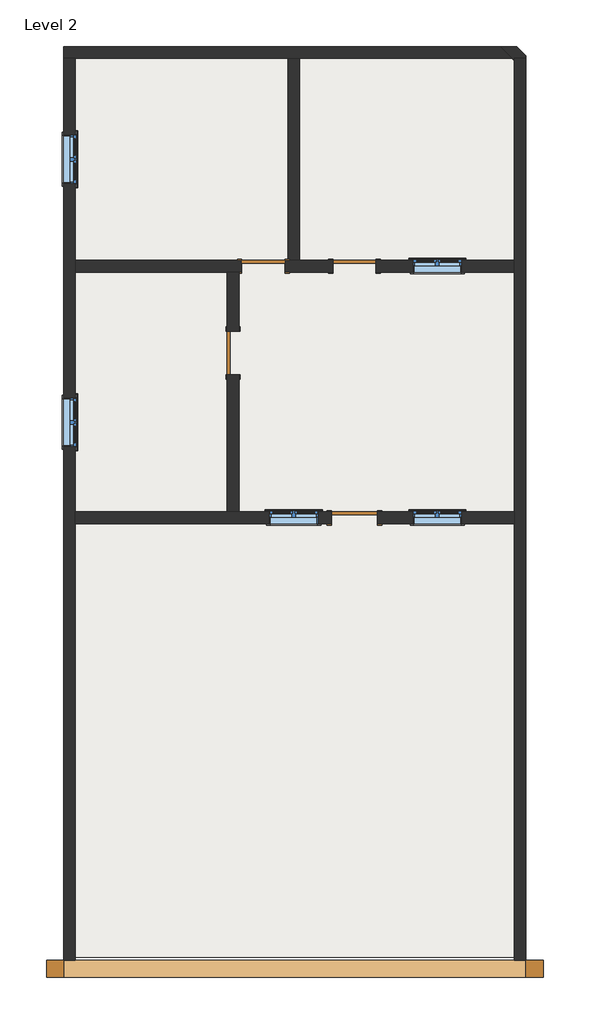
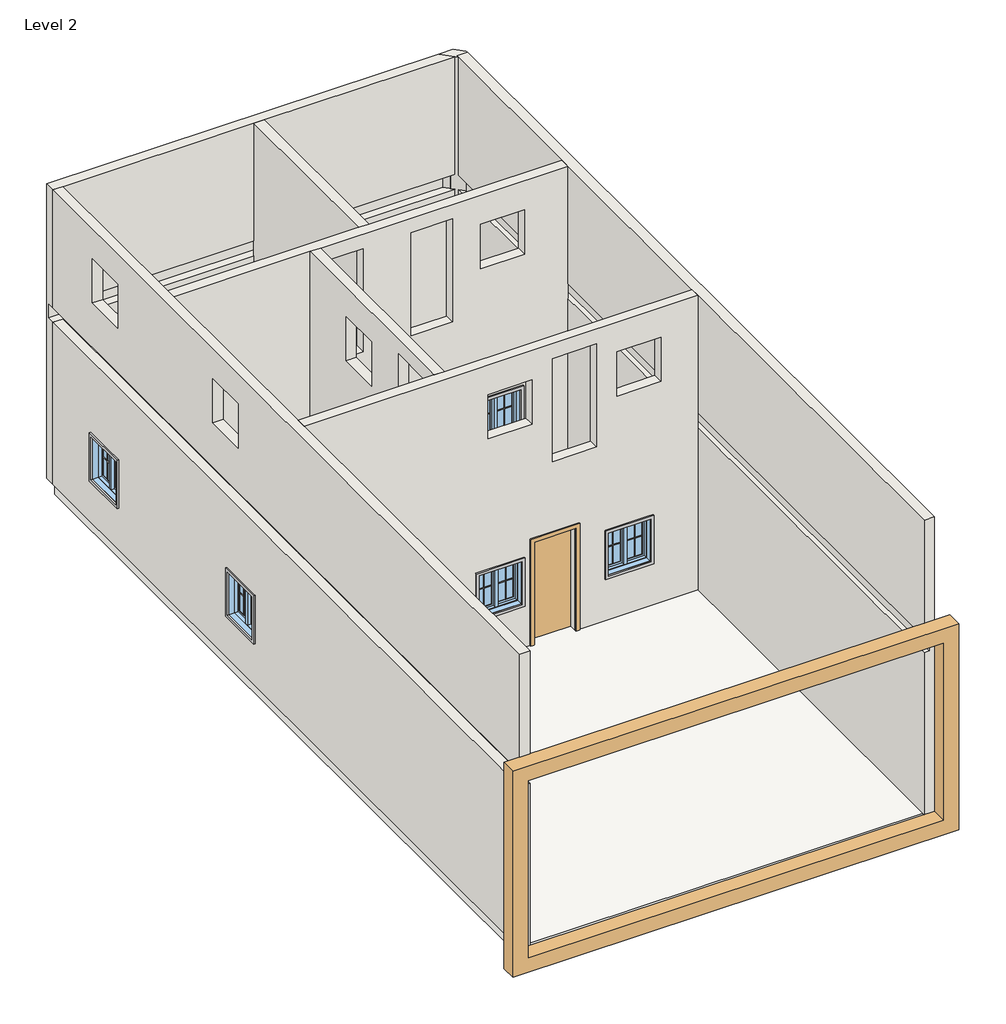
# One storey: 20 proxies, 8 walls, 5 doors, 5 windows, 1 slab.
"""IFC4 building model written with IfcOpenShell, lengths in millimetres."""

from ifc_helpers import new_model, si_unit, frame, origin, place, context, project, spatial, polyline, outline, extrude, faceted_brep, transform, mapped, element, save
from components import muntin_pattern_2x2_muntin_pattern_2x2_b3fe6957, muntin_pattern_2x2_muntin_pattern_2x2_3e0ecaf2, trim_window_exterior_flat_with_sill_41619996, trim_window_interior_flat_picture_frame_51c85655, doors_1_doors_1_af7bef9e, door_fadea3f2, door_64d5ae29, window_c29befe5

model = new_model("IFC4")

# Units and contexts
model_context = context("Model", 3, world=origin())
ifc_project = project(units=[si_unit("LENGTHUNIT", "METRE", prefix="MILLI")], contexts=[model_context])

# Site, building, storey
site = spatial("IfcSite", under=ifc_project)
building = spatial("IfcBuilding", under=site)
storey = spatial("IfcBuildingStorey", under=building, Name="Level 2", Elevation=9144.0)

# Proxies
placement = place(None, origin())
muntin_pattern_2x2_muntin_pattern_2x2_shape = muntin_pattern_2x2_muntin_pattern_2x2_b3fe6957(model_context)
element("IfcBuildingElementProxy", 1, Name="Muntin Pattern_2x2 : Muntin Pattern_2x2", ObjectType="Muntin Pattern_2x2 : Muntin Pattern_2x2", at=placement, inside=storey, context=model_context, shape_type="MappedRepresentation", body=[
    mapped(muntin_pattern_2x2_muntin_pattern_2x2_shape, transform((-9669.8723431, 12327.0201951, 10128.25), x_axis=(1.0, 0.0, 0.0), y_axis=(0.0, 1.0, 0.0), z_axis=(0.0, 0.0, 1.0))),
])
element("IfcBuildingElementProxy", 2, Name="Muntin Pattern_2x2 : Muntin Pattern_2x2", ObjectType="Muntin Pattern_2x2 : Muntin Pattern_2x2", at=placement, inside=storey, context=model_context, shape_type="MappedRepresentation", body=[
    mapped(muntin_pattern_2x2_muntin_pattern_2x2_shape, transform((-15829.9638186, 14328.8576951, 10128.25), x_axis=(0.0, -1.0, 0.0), y_axis=(1.0, 0.0, 0.0), z_axis=(0.0, 0.0, 1.0))),
])
element("IfcBuildingElementProxy", 3, Name="Muntin Pattern_2x2 : Muntin Pattern_2x2", ObjectType="Muntin Pattern_2x2 : Muntin Pattern_2x2", at=placement, inside=storey, context=model_context, shape_type="MappedRepresentation", body=[
    mapped(muntin_pattern_2x2_muntin_pattern_2x2_shape, transform((-15829.9638186, 9706.0576951, 10128.25), x_axis=(0.0, -1.0, 0.0), y_axis=(1.0, 0.0, 0.0), z_axis=(0.0, 0.0, 1.0))),
])
element("IfcBuildingElementProxy", 4, Name="Muntin Pattern_2x2 : Muntin Pattern_2x2", ObjectType="Muntin Pattern_2x2 : Muntin Pattern_2x2", at=placement, inside=storey, context=model_context, shape_type="MappedRepresentation", body=[
    mapped(muntin_pattern_2x2_muntin_pattern_2x2_shape, transform((-12194.9933676, 7907.4201951, 10128.25), x_axis=(1.0, 0.0, 0.0), y_axis=(0.0, 1.0, 0.0), z_axis=(0.0, 0.0, 1.0))),
])
element("IfcBuildingElementProxy", 5, Name="Muntin Pattern_2x2 : Muntin Pattern_2x2", ObjectType="Muntin Pattern_2x2 : Muntin Pattern_2x2", at=placement, inside=storey, context=model_context, shape_type="MappedRepresentation", body=[
    mapped(muntin_pattern_2x2_muntin_pattern_2x2_shape, transform((-9669.8723431, 7907.4201951, 10128.25), x_axis=(1.0, 0.0, 0.0), y_axis=(0.0, 1.0, 0.0), z_axis=(0.0, 0.0, 1.0))),
])
muntin_pattern_2x2_muntin_pattern_2x2_2_shape = muntin_pattern_2x2_muntin_pattern_2x2_3e0ecaf2(model_context)
element("IfcBuildingElementProxy", 6, Name="Muntin Pattern_2x2 : Muntin Pattern_2x2", ObjectType="Muntin Pattern_2x2 : Muntin Pattern_2x2", at=placement, inside=storey, context=model_context, shape_type="MappedRepresentation", body=[
    mapped(muntin_pattern_2x2_muntin_pattern_2x2_2_shape, transform((-9241.2473431, 12327.0201951, 10128.25), x_axis=(-1.0, 0.0, 0.0), y_axis=(0.0, -1.0, 0.0), z_axis=(0.0, 0.0, 1.0))),
])
element("IfcBuildingElementProxy", 7, Name="Muntin Pattern_2x2 : Muntin Pattern_2x2", ObjectType="Muntin Pattern_2x2 : Muntin Pattern_2x2", at=placement, inside=storey, context=model_context, shape_type="MappedRepresentation", body=[
    mapped(muntin_pattern_2x2_muntin_pattern_2x2_2_shape, transform((-15829.9638186, 13900.2326951, 10128.25), x_axis=(0.0, 1.0, 0.0), y_axis=(-1.0, 0.0, 0.0), z_axis=(0.0, 0.0, 1.0))),
])
element("IfcBuildingElementProxy", 8, Name="Muntin Pattern_2x2 : Muntin Pattern_2x2", ObjectType="Muntin Pattern_2x2 : Muntin Pattern_2x2", at=placement, inside=storey, context=model_context, shape_type="MappedRepresentation", body=[
    mapped(muntin_pattern_2x2_muntin_pattern_2x2_2_shape, transform((-15829.9638186, 9277.4326951, 10128.25), x_axis=(0.0, 1.0, 0.0), y_axis=(-1.0, 0.0, 0.0), z_axis=(0.0, 0.0, 1.0))),
])
element("IfcBuildingElementProxy", 9, Name="Muntin Pattern_2x2 : Muntin Pattern_2x2", ObjectType="Muntin Pattern_2x2 : Muntin Pattern_2x2", at=placement, inside=storey, context=model_context, shape_type="MappedRepresentation", body=[
    mapped(muntin_pattern_2x2_muntin_pattern_2x2_2_shape, transform((-11766.3683676, 7907.4201951, 10128.25), x_axis=(-1.0, 0.0, 0.0), y_axis=(0.0, -1.0, 0.0), z_axis=(0.0, 0.0, 1.0))),
])
element("IfcBuildingElementProxy", 10, Name="Muntin Pattern_2x2 : Muntin Pattern_2x2", ObjectType="Muntin Pattern_2x2 : Muntin Pattern_2x2", at=placement, inside=storey, context=model_context, shape_type="MappedRepresentation", body=[
    mapped(muntin_pattern_2x2_muntin_pattern_2x2_2_shape, transform((-9241.2473431, 7907.4201951, 10128.25), x_axis=(-1.0, 0.0, 0.0), y_axis=(0.0, -1.0, 0.0), z_axis=(0.0, 0.0, 1.0))),
])
trim_window_exterior_flat_with_sill_shape = trim_window_exterior_flat_with_sill_41619996(model_context)
element("IfcBuildingElementProxy", 11, Name="Trim-Window-Exterior-Flat : with Sill", ObjectType="Trim-Window-Exterior-Flat : with Sill", at=placement, inside=storey, context=model_context, shape_type="MappedRepresentation", body=[
    mapped(trim_window_exterior_flat_with_sill_shape, transform((-9455.5598431, 12336.5451951, 10972.8), x_axis=(-1.0, 0.0, 0.0), y_axis=(0.0, 0.0, 1.0), z_axis=(0.0, 1.0, 0.0))),
])
element("IfcBuildingElementProxy", 12, Name="Trim-Window-Exterior-Flat : with Sill", ObjectType="Trim-Window-Exterior-Flat : with Sill", at=placement, inside=storey, context=model_context, shape_type="MappedRepresentation", body=[
    mapped(trim_window_exterior_flat_with_sill_shape, transform((-15820.4388186, 14114.5451951, 10972.8), x_axis=(0.0, 1.0, 0.0), y_axis=(0.0, 0.0, 1.0), z_axis=(1.0, 0.0, 0.0))),
])
element("IfcBuildingElementProxy", 13, Name="Trim-Window-Exterior-Flat : with Sill", ObjectType="Trim-Window-Exterior-Flat : with Sill", at=placement, inside=storey, context=model_context, shape_type="MappedRepresentation", body=[
    mapped(trim_window_exterior_flat_with_sill_shape, transform((-15820.4388186, 9491.7451951, 10972.8), x_axis=(0.0, 1.0, 0.0), y_axis=(0.0, 0.0, 1.0), z_axis=(1.0, 0.0, 0.0))),
])
element("IfcBuildingElementProxy", 14, Name="Trim-Window-Exterior-Flat : with Sill", ObjectType="Trim-Window-Exterior-Flat : with Sill", at=placement, inside=storey, context=model_context, shape_type="MappedRepresentation", body=[
    mapped(trim_window_exterior_flat_with_sill_shape, transform((-11980.6808676, 7916.9451951, 10972.8), x_axis=(-1.0, 0.0, 0.0), y_axis=(0.0, 0.0, 1.0), z_axis=(0.0, 1.0, 0.0))),
])
element("IfcBuildingElementProxy", 15, Name="Trim-Window-Exterior-Flat : with Sill", ObjectType="Trim-Window-Exterior-Flat : with Sill", at=placement, inside=storey, context=model_context, shape_type="MappedRepresentation", body=[
    mapped(trim_window_exterior_flat_with_sill_shape, transform((-9455.5598431, 7916.9451951, 10972.8), x_axis=(-1.0, 0.0, 0.0), y_axis=(0.0, 0.0, 1.0), z_axis=(0.0, 1.0, 0.0))),
])
trim_window_interior_flat_picture_frame_shape = trim_window_interior_flat_picture_frame_51c85655(model_context)
element("IfcBuildingElementProxy", 16, Name="Trim-Window-Interior-Flat : Picture Frame", ObjectType="Trim-Window-Interior-Flat : Picture Frame", at=placement, inside=storey, context=model_context, shape_type="MappedRepresentation", body=[
    mapped(trim_window_interior_flat_picture_frame_shape, transform((-9455.5598431, 12133.3451951, 10972.8), x_axis=(1.0, 0.0, 0.0), y_axis=(0.0, 0.0, 1.0), z_axis=(0.0, -1.0, 0.0))),
])
element("IfcBuildingElementProxy", 17, Name="Trim-Window-Interior-Flat : Picture Frame", ObjectType="Trim-Window-Interior-Flat : Picture Frame", at=placement, inside=storey, context=model_context, shape_type="MappedRepresentation", body=[
    mapped(trim_window_interior_flat_picture_frame_shape, transform((-16023.6388186, 14114.5451951, 10972.8), x_axis=(0.0, -1.0, 0.0), y_axis=(0.0, 0.0, 1.0), z_axis=(-1.0, 0.0, 0.0))),
])
element("IfcBuildingElementProxy", 18, Name="Trim-Window-Interior-Flat : Picture Frame", ObjectType="Trim-Window-Interior-Flat : Picture Frame", at=placement, inside=storey, context=model_context, shape_type="MappedRepresentation", body=[
    mapped(trim_window_interior_flat_picture_frame_shape, transform((-16023.6388186, 9491.7451951, 10972.8), x_axis=(0.0, -1.0, 0.0), y_axis=(0.0, 0.0, 1.0), z_axis=(-1.0, 0.0, 0.0))),
])
element("IfcBuildingElementProxy", 19, Name="Trim-Window-Interior-Flat : Picture Frame", ObjectType="Trim-Window-Interior-Flat : Picture Frame", at=placement, inside=storey, context=model_context, shape_type="MappedRepresentation", body=[
    mapped(trim_window_interior_flat_picture_frame_shape, transform((-11980.6808676, 7713.7451951, 10972.8), x_axis=(1.0, 0.0, 0.0), y_axis=(0.0, 0.0, 1.0), z_axis=(0.0, -1.0, 0.0))),
])
element("IfcBuildingElementProxy", 20, Name="Trim-Window-Interior-Flat : Picture Frame", ObjectType="Trim-Window-Interior-Flat : Picture Frame", at=placement, inside=storey, context=model_context, shape_type="MappedRepresentation", body=[
    mapped(trim_window_interior_flat_picture_frame_shape, transform((-9455.5598431, 7713.7451951, 10972.8), x_axis=(1.0, 0.0, 0.0), y_axis=(0.0, 0.0, 1.0), z_axis=(0.0, -1.0, 0.0))),
])

# Doors
doors_1_doors_1_shape = doors_1_doors_1_af7bef9e(model_context)
element("IfcDoor", 21, ObjectType="Doors 1 : Doors 1", at=placement, inside=storey, context=model_context, shape_type="MappedRepresentation", body=[
    mapped(doors_1_doors_1_shape, transform((0.0, 0.0, 0.0), x_axis=(1.0, 0.0, 0.0), y_axis=(0.0, 1.0, 0.0), z_axis=(0.0, 0.0, 1.0))),
])
door_shape = door_fadea3f2(model_context)
element("IfcDoor", 22, ObjectType="Single-Flush : 30\" x 80\"", at=placement, inside=storey, context=model_context, shape_type="MappedRepresentation", body=[
    mapped(door_shape, transform((-12514.0808676, 12234.9451951, 9144.0), x_axis=(1.0, 0.0, 0.0), y_axis=(0.0, 1.0, 0.0), z_axis=(0.0, 0.0, 1.0))),
])
element("IfcDoor", 23, ObjectType="Single-Flush : 30\" x 80\"", at=placement, inside=storey, context=model_context, shape_type="MappedRepresentation", body=[
    mapped(door_shape, transform((-10913.8808676, 12234.9451951, 9144.0), x_axis=(1.0, 0.0, 0.0), y_axis=(0.0, 1.0, 0.0), z_axis=(0.0, 0.0, 1.0))),
])
element("IfcDoor", 24, ObjectType="Single-Flush : 30\" x 80\"", at=placement, inside=storey, context=model_context, shape_type="MappedRepresentation", body=[
    mapped(door_shape, transform((-13047.4808676, 10710.9451951, 9144.0), x_axis=(0.0, 1.0, 0.0), y_axis=(-1.0, 0.0, 0.0), z_axis=(0.0, 0.0, 1.0))),
])
door_2_shape = door_64d5ae29(model_context)
element("IfcDoor", 25, ObjectType="Single-Flush : 32\" x 84\"", at=placement, inside=storey, context=model_context, shape_type="MappedRepresentation", body=[
    mapped(door_2_shape, transform((-10913.8808676, 7815.3451951, 9144.0), x_axis=(1.0, 0.0, 0.0), y_axis=(0.0, 1.0, 0.0), z_axis=(0.0, 0.0, 1.0))),
])

# Slab
element("IfcSlab", 26, ObjectType="Generic - 12\"", at=placement, inside=storey, context=model_context, shape_type="SweptSolid", body=[
    extrude(outline(polyline([(-8098.8388186, 15994.1451951), (-8098.8388186, 93.7451951), (-15922.0388186, 93.7451951), (-15922.0388186, 15994.1451951), (-8098.8388186, 15994.1451951)])), frame((0.0, 0.0, 8839.2), z_axis=(0.0, 0.0, 1.0), x_axis=(1.0, 0.0, 0.0)), (0.0, 0.0, 1.0), 304.8),
])

# Walls
element("IfcWall", 27, ObjectType="Generic - 8\" - Filled", at=placement, inside=storey, context=model_context, shape_type="Brep", body=[
    faceted_brep([(-16023.6388186, 15892.5451951, 9144.0), (-15820.4388186, 15892.5451951, 9144.0), (-12082.2808676, 15892.5451951, 9144.0), (-11879.0808676, 15892.5451951, 9144.0), (-8140.9229165, 15892.5451951, 9144.0), (-8140.9229165, 15892.5451951, 12496.8), (-15820.4388186, 15892.5451951, 12496.8), (-16023.6388186, 15892.5451951, 12496.8), (-8140.9229165, 15892.5451951, 15240.0), (-11879.0808676, 15892.5451951, 15240.0), (-12082.2808676, 15892.5451951, 15240.0), (-15820.4388186, 15892.5451951, 15240.0), (-16023.6388186, 15892.5451951, 15240.0), (-16023.6388186, 15892.5451951, 12801.6), (-15820.4388186, 15892.5451951, 12801.6), (-8140.9229165, 15892.5451951, 12801.6), (-8344.1229165, 16095.7451951, 9144.0), (-16023.6388186, 16095.7451951, 9144.0), (-16023.6388186, 16095.7451951, 15240.0), (-8344.1229165, 16095.7451951, 15240.0), (-8191.7229165, 15943.3451951, 12801.6), (-8191.7229165, 15943.3451951, 12496.8), (-8293.3229165, 16044.9451951, 12496.8), (-8200.4388186, 15952.0610972, 12496.8), (-8200.4388186, 15952.0610972, 12801.6), (-8293.3229165, 16044.9451951, 12801.6), (-16023.6388186, 16044.9451951, 12496.8), (-16023.6388186, 16044.9451951, 12801.6), (-8200.4388186, 15943.3451951, 12496.8), (-8200.4388186, 15943.3451951, 12801.6)], [[[0, 1, 2, 3, 4, 5, 6, 7]], [[8, 9, 10, 11, 12, 13, 14, 15]], [[16, 17, 18, 19]], [[4, 3, 2, 1, 0, 17, 16]], [[12, 11, 10, 9, 8, 19, 18]], [[4, 16, 19, 8, 15, 20, 21, 5], [22, 23, 24, 25]], [[12, 18, 17, 0, 7, 26, 27, 13]], [[5, 21, 28, 23, 22, 26, 7, 6]], [[20, 15, 14, 13, 27, 25, 24, 29]], [[21, 20, 29, 28]], [[23, 28, 29, 24]], [[26, 22, 25, 27]]]),
])
element("IfcWall", 28, ObjectType="Generic - 8\" - Filled", at=placement, inside=storey, context=model_context, shape_type="Brep", body=[
    faceted_brep([(-8344.1229165, 16095.7451951, 9144.0), (-8140.9229165, 15892.5451951, 9144.0), (-7895.6388186, 15647.2610972, 9144.0), (-7895.6388186, 15647.2610972, 15240.0), (-8140.9229165, 15892.5451951, 15240.0), (-8344.1229165, 16095.7451951, 15240.0), (-8056.7547207, 16095.7451951, 9144.0), (-8056.7547207, 16095.7451951, 15240.0), (-7895.6388186, 15934.6292931, 15240.0), (-7895.6388186, 15934.6292931, 9144.0)], [[[0, 1, 2, 3, 4, 5]], [[6, 7, 8, 9]], [[2, 1, 0, 6, 9]], [[5, 4, 3, 8, 7]], [[0, 5, 7, 6]], [[3, 2, 9, 8]]]),
])
element("IfcWall", 29, ObjectType="Generic - 8\" - Filled", at=placement, inside=storey, context=model_context, shape_type="Brep", body=[
    faceted_brep([(-8098.8388186, 15892.5451951, 9144.0), (-8098.8388186, 12336.5451951, 9144.0), (-8098.8388186, 12133.3451951, 9144.0), (-8098.8388186, 7916.9451951, 9144.0), (-8098.8388186, 7713.7451951, 9144.0), (-8098.8388186, 42.9451951, 9144.0), (-8098.8388186, 42.9451951, 12496.8), (-8098.8388186, 15892.5451951, 12496.8), (-8098.8388186, 42.9451951, 15240.0), (-8098.8388186, 7713.7451951, 15240.0), (-8098.8388186, 7916.9451951, 15240.0), (-8098.8388186, 12133.3451951, 15240.0), (-8098.8388186, 12336.5451951, 15240.0), (-8098.8388186, 15892.5451951, 15240.0), (-8098.8388186, 15892.5451951, 12801.6), (-8098.8388186, 42.9451951, 12801.6), (-7895.6388186, 42.9451951, 9144.0), (-7895.6388186, 15892.5451951, 9144.0), (-7895.6388186, 15892.5451951, 15240.0), (-7895.6388186, 42.9451951, 15240.0), (-7997.2388186, 42.9451951, 12801.6), (-7997.2388186, 42.9451951, 12496.8), (-7997.2388186, 15892.5451951, 12496.8), (-7997.2388186, 15892.5451951, 12801.6)], [[[0, 1, 2, 3, 4, 5, 6, 7]], [[8, 9, 10, 11, 12, 13, 14, 15]], [[16, 17, 18, 19]], [[5, 4, 3, 2, 1, 0, 17, 16]], [[16, 19, 8, 15, 20, 21, 6, 5]], [[13, 12, 11, 10, 9, 8, 19, 18]], [[13, 18, 17, 0, 7, 22, 23, 14]], [[21, 22, 7, 6]], [[23, 20, 15, 14]], [[22, 21, 20, 23]]]),
])
element("IfcWall", 30, ObjectType="Generic - 8\" - Filled", at=placement, inside=storey, context=model_context, shape_type="Brep", body=[
    faceted_brep([(-15820.4388186, 15892.5451951, 15240.0), (-15820.4388186, 12336.5451951, 15240.0), (-15820.4388186, 12133.3451951, 15240.0), (-15820.4388186, 7916.9451951, 15240.0), (-15820.4388186, 7713.7451951, 15240.0), (-15820.4388186, 42.9451951, 15240.0), (-15820.4388186, 42.9451951, 12801.6), (-15820.4388186, 15892.5451951, 12801.6), (-15820.4388186, 13682.7451951, 13716.0), (-15820.4388186, 13682.7451951, 14630.4), (-15820.4388186, 14546.3451951, 14630.4), (-15820.4388186, 14546.3451951, 13716.0), (-15820.4388186, 9593.3451951, 13716.0), (-15820.4388186, 9593.3451951, 14630.4), (-15820.4388186, 10456.9451951, 14630.4), (-15820.4388186, 10456.9451951, 13716.0), (-16023.6388186, 42.9451951, 15240.0), (-16023.6388186, 15892.5451951, 15240.0), (-16023.6388186, 15892.5451951, 12801.6), (-16023.6388186, 42.9451951, 12801.6), (-16023.6388186, 13682.7451951, 14630.4), (-16023.6388186, 13682.7451951, 13716.0), (-16023.6388186, 14546.3451951, 13716.0), (-16023.6388186, 14546.3451951, 14630.4), (-16023.6388186, 9593.3451951, 14630.4), (-16023.6388186, 9593.3451951, 13716.0), (-16023.6388186, 10456.9451951, 13716.0), (-16023.6388186, 10456.9451951, 14630.4)], [[[0, 1, 2, 3, 4, 5, 6, 7], [8, 9, 10, 11], [12, 13, 14, 15]], [[16, 17, 18, 19], [20, 21, 22, 23], [24, 25, 26, 27]], [[5, 4, 3, 2, 1, 0, 17, 16]], [[5, 16, 19, 6]], [[17, 0, 7, 18]], [[21, 20, 9, 8]], [[22, 21, 8, 11]], [[23, 22, 11, 10]], [[20, 23, 10, 9]], [[25, 24, 13, 12]], [[26, 25, 12, 15]], [[27, 26, 15, 14]], [[24, 27, 14, 13]], [[7, 6, 19, 18]]]),
    faceted_brep([(-15820.4388186, 42.9451951, 9144.0), (-15820.4388186, 7713.7451951, 9144.0), (-15820.4388186, 7916.9451951, 9144.0), (-15820.4388186, 12133.3451951, 9144.0), (-15820.4388186, 12336.5451951, 9144.0), (-15820.4388186, 15892.5451951, 9144.0), (-15820.4388186, 15892.5451951, 12496.8), (-15820.4388186, 42.9451951, 12496.8), (-15820.4388186, 13682.7451951, 10058.4), (-15820.4388186, 13682.7451951, 10972.8), (-15820.4388186, 14546.3451951, 10972.8), (-15820.4388186, 14546.3451951, 10058.4), (-15820.4388186, 9059.9451951, 10058.4), (-15820.4388186, 9059.9451951, 10972.8), (-15820.4388186, 9923.5451951, 10972.8), (-15820.4388186, 9923.5451951, 10058.4), (-16023.6388186, 15892.5451951, 9144.0), (-16023.6388186, 42.9451951, 9144.0), (-16023.6388186, 42.9451951, 12496.8), (-16023.6388186, 15892.5451951, 12496.8), (-16023.6388186, 13682.7451951, 10972.8), (-16023.6388186, 13682.7451951, 10058.4), (-16023.6388186, 14546.3451951, 10058.4), (-16023.6388186, 14546.3451951, 10972.8), (-16023.6388186, 9059.9451951, 10972.8), (-16023.6388186, 9059.9451951, 10058.4), (-16023.6388186, 9923.5451951, 10058.4), (-16023.6388186, 9923.5451951, 10972.8)], [[[0, 1, 2, 3, 4, 5, 6, 7], [8, 9, 10, 11], [12, 13, 14, 15]], [[16, 17, 18, 19], [20, 21, 22, 23], [24, 25, 26, 27]], [[5, 4, 3, 2, 1, 0, 17, 16]], [[17, 0, 7, 18]], [[5, 16, 19, 6]], [[21, 20, 9, 8]], [[22, 21, 8, 11]], [[23, 22, 11, 10]], [[20, 23, 10, 9]], [[25, 24, 13, 12]], [[26, 25, 12, 15]], [[27, 26, 15, 14]], [[24, 27, 14, 13]], [[7, 6, 19, 18]]]),
])
element("IfcWall", 31, ObjectType="Generic - 8\" - Filled", at=placement, inside=storey, context=model_context, shape_type="SweptSolid", body=[
    extrude(outline(polyline([(-12082.2808676, 12336.5451951), (-12082.2808676, 15892.5451951), (-11879.0808676, 15892.5451951), (-11879.0808676, 12336.5451951), (-12082.2808676, 12336.5451951)])), frame((0.0, 0.0, 9144.0), z_axis=(0.0, 0.0, 1.0), x_axis=(1.0, 0.0, 0.0)), (0.0, 0.0, 1.0), 6096.0),
])
element("IfcWall", 32, ObjectType="Generic - 8\" - Filled", at=placement, inside=storey, context=model_context, shape_type="Brep", body=[
    faceted_brep([(-8098.8388186, 12336.5451951, 9144.0), (-10532.8808676, 12336.5451951, 9144.0), (-10532.8808676, 12336.5451951, 11176.0), (-11294.8808676, 12336.5451951, 11176.0), (-11294.8808676, 12336.5451951, 9144.0), (-11879.0808676, 12336.5451951, 9144.0), (-12082.2808676, 12336.5451951, 9144.0), (-12133.0808676, 12336.5451951, 9144.0), (-12133.0808676, 12336.5451951, 11176.0), (-12895.0808676, 12336.5451951, 11176.0), (-12895.0808676, 12336.5451951, 9144.0), (-15820.4388186, 12336.5451951, 9144.0), (-15820.4388186, 12336.5451951, 15240.0), (-12082.2808676, 12336.5451951, 15240.0), (-11879.0808676, 12336.5451951, 15240.0), (-8098.8388186, 12336.5451951, 15240.0), (-9023.7598431, 12336.5451951, 10972.8), (-9887.3598431, 12336.5451951, 10972.8), (-9887.3598431, 12336.5451951, 10058.4), (-9023.7598431, 12336.5451951, 10058.4), (-12920.4808676, 12336.5451951, 12801.6), (-12107.6808676, 12336.5451951, 12801.6), (-12107.6808676, 12336.5451951, 14935.2), (-12920.4808676, 12336.5451951, 14935.2), (-11167.8808676, 12336.5451951, 12801.6), (-10355.0808676, 12336.5451951, 12801.6), (-10355.0808676, 12336.5451951, 14935.2), (-11167.8808676, 12336.5451951, 14935.2), (-8947.5598431, 12336.5451951, 14630.4), (-9811.1598431, 12336.5451951, 14630.4), (-9811.1598431, 12336.5451951, 13716.0), (-8947.5598431, 12336.5451951, 13716.0), (-10532.8808676, 12133.3451951, 11176.0), (-10532.8808676, 12133.3451951, 9144.0), (-8098.8388186, 12133.3451951, 9144.0), (-8098.8388186, 12133.3451951, 15240.0), (-12945.8808676, 12133.3451951, 15240.0), (-13149.0808676, 12133.3451951, 15240.0), (-15820.4388186, 12133.3451951, 15240.0), (-15820.4388186, 12133.3451951, 9144.0), (-13149.0808676, 12133.3451951, 9144.0), (-12945.8808676, 12133.3451951, 9144.0), (-12895.0808676, 12133.3451951, 9144.0), (-12895.0808676, 12133.3451951, 11176.0), (-12133.0808676, 12133.3451951, 11176.0), (-12133.0808676, 12133.3451951, 9144.0), (-11294.8808676, 12133.3451951, 9144.0), (-11294.8808676, 12133.3451951, 11176.0), (-9023.7598431, 12133.3451951, 10972.8), (-9023.7598431, 12133.3451951, 10058.4), (-9887.3598431, 12133.3451951, 10058.4), (-9887.3598431, 12133.3451951, 10972.8), (-12920.4808676, 12133.3451951, 12801.6), (-12920.4808676, 12133.3451951, 14935.2), (-12107.6808676, 12133.3451951, 14935.2), (-12107.6808676, 12133.3451951, 12801.6), (-11167.8808676, 12133.3451951, 12801.6), (-11167.8808676, 12133.3451951, 14935.2), (-10355.0808676, 12133.3451951, 14935.2), (-10355.0808676, 12133.3451951, 12801.6), (-8947.5598431, 12133.3451951, 14630.4), (-8947.5598431, 12133.3451951, 13716.0), (-9811.1598431, 12133.3451951, 13716.0), (-9811.1598431, 12133.3451951, 14630.4)], [[[0, 1, 2, 3, 4, 5, 6, 7, 8, 9, 10, 11, 12, 13, 14, 15], [16, 17, 18, 19], [20, 21, 22, 23], [24, 25, 26, 27], [28, 29, 30, 31]], [[32, 33, 34, 35, 36, 37, 38, 39, 40, 41, 42, 43, 44, 45, 46, 47], [48, 49, 50, 51], [52, 53, 54, 55], [56, 57, 58, 59], [60, 61, 62, 63]], [[42, 41, 40, 39, 11, 10]], [[46, 45, 7, 6, 5, 4]], [[34, 33, 1, 0]], [[15, 14, 13, 12, 38, 37, 36, 35]], [[12, 11, 39, 38]], [[0, 15, 35, 34]], [[8, 7, 45, 44]], [[9, 8, 44, 43]], [[10, 9, 43, 42]], [[2, 1, 33, 32]], [[3, 2, 32, 47]], [[4, 3, 47, 46]], [[49, 48, 16, 19]], [[50, 49, 19, 18]], [[51, 50, 18, 17]], [[48, 51, 17, 16]], [[21, 20, 52, 55]], [[22, 21, 55, 54]], [[23, 22, 54, 53]], [[20, 23, 53, 52]], [[25, 24, 56, 59]], [[26, 25, 59, 58]], [[27, 26, 58, 57]], [[24, 27, 57, 56]], [[61, 60, 28, 31]], [[62, 61, 31, 30]], [[63, 62, 30, 29]], [[60, 63, 29, 28]]]),
])
element("IfcWall", 33, ObjectType="Generic - 8\" - Filled", at=placement, inside=storey, context=model_context, shape_type="SweptSolid", body=[
    extrude(outline(polyline([(12133.3451951, 9144.0), (11091.9451951, 9144.0), (11091.9451951, 11176.0), (10329.9451951, 11176.0), (10329.9451951, 9144.0), (7916.9451951, 9144.0), (7916.9451951, 15240.0), (12133.3451951, 15240.0), (12133.3451951, 9144.0)]), holes=[polyline([(8323.3451951, 12801.6), (9136.1451951, 12801.6), (9136.1451951, 14935.2), (8323.3451951, 14935.2), (8323.3451951, 12801.6)]), polyline([(10914.1451951, 14630.4), (10050.5451951, 14630.4), (10050.5451951, 13716.0), (10914.1451951, 13716.0), (10914.1451951, 14630.4)])]), frame((-13149.0808676, 0.0, 0.0), z_axis=(1.0, 0.0, 0.0), x_axis=(0.0, 1.0, 0.0)), (0.0, 0.0, 1.0), 203.2),
])
element("IfcWall", 34, ObjectType="Generic - 8\" - Filled", at=placement, inside=storey, context=model_context, shape_type="Brep", body=[
    faceted_brep([(-8098.8388186, 7916.9451951, 9144.0), (-10507.4808676, 7916.9451951, 9144.0), (-10507.4808676, 7916.9451951, 11277.6), (-11320.2808676, 7916.9451951, 11277.6), (-11320.2808676, 7916.9451951, 9144.0), (-12945.8808676, 7916.9451951, 9144.0), (-13149.0808676, 7916.9451951, 9144.0), (-15820.4388186, 7916.9451951, 9144.0), (-15820.4388186, 7916.9451951, 15240.0), (-13149.0808676, 7916.9451951, 15240.0), (-12945.8808676, 7916.9451951, 15240.0), (-8098.8388186, 7916.9451951, 15240.0), (-10954.1598431, 7916.9451951, 12801.6), (-10090.5598431, 7916.9451951, 12801.6), (-10090.5598431, 7916.9451951, 14935.2), (-10954.1598431, 7916.9451951, 14935.2), (-8827.9993308, 7916.9451951, 14630.4), (-9691.5993308, 7916.9451951, 14630.4), (-9691.5993308, 7916.9451951, 13716.0), (-8827.9993308, 7916.9451951, 13716.0), (-11353.1203553, 7916.9451951, 14630.4), (-12216.7203553, 7916.9451951, 14630.4), (-12216.7203553, 7916.9451951, 13716.0), (-11353.1203553, 7916.9451951, 13716.0), (-11548.8808676, 7916.9451951, 10972.8), (-12412.4808676, 7916.9451951, 10972.8), (-12412.4808676, 7916.9451951, 10058.4), (-11548.8808676, 7916.9451951, 10058.4), (-9023.7598431, 7916.9451951, 10972.8), (-9887.3598431, 7916.9451951, 10972.8), (-9887.3598431, 7916.9451951, 10058.4), (-9023.7598431, 7916.9451951, 10058.4), (-10507.4808676, 7713.7451951, 11277.6), (-10507.4808676, 7713.7451951, 9144.0), (-8098.8388186, 7713.7451951, 9144.0), (-8098.8388186, 7713.7451951, 15240.0), (-15820.4388186, 7713.7451951, 15240.0), (-15820.4388186, 7713.7451951, 9144.0), (-11320.2808676, 7713.7451951, 9144.0), (-11320.2808676, 7713.7451951, 11277.6), (-10954.1598431, 7713.7451951, 12801.6), (-10954.1598431, 7713.7451951, 14935.2), (-10090.5598431, 7713.7451951, 14935.2), (-10090.5598431, 7713.7451951, 12801.6), (-8827.9993308, 7713.7451951, 14630.4), (-8827.9993308, 7713.7451951, 13716.0), (-9691.5993308, 7713.7451951, 13716.0), (-9691.5993308, 7713.7451951, 14630.4), (-11353.1203553, 7713.7451951, 14630.4), (-11353.1203553, 7713.7451951, 13716.0), (-12216.7203553, 7713.7451951, 13716.0), (-12216.7203553, 7713.7451951, 14630.4), (-11548.8808676, 7713.7451951, 10972.8), (-11548.8808676, 7713.7451951, 10058.4), (-12412.4808676, 7713.7451951, 10058.4), (-12412.4808676, 7713.7451951, 10972.8), (-9023.7598431, 7713.7451951, 10972.8), (-9023.7598431, 7713.7451951, 10058.4), (-9887.3598431, 7713.7451951, 10058.4), (-9887.3598431, 7713.7451951, 10972.8)], [[[0, 1, 2, 3, 4, 5, 6, 7, 8, 9, 10, 11], [12, 13, 14, 15], [16, 17, 18, 19], [20, 21, 22, 23], [24, 25, 26, 27], [28, 29, 30, 31]], [[32, 33, 34, 35, 36, 37, 38, 39], [40, 41, 42, 43], [44, 45, 46, 47], [48, 49, 50, 51], [52, 53, 54, 55], [56, 57, 58, 59]], [[38, 37, 7, 6, 5, 4]], [[34, 33, 1, 0]], [[11, 10, 9, 8, 36, 35]], [[8, 7, 37, 36]], [[0, 11, 35, 34]], [[2, 1, 33, 32]], [[3, 2, 32, 39]], [[4, 3, 39, 38]], [[13, 12, 40, 43]], [[14, 13, 43, 42]], [[15, 14, 42, 41]], [[12, 15, 41, 40]], [[45, 44, 16, 19]], [[46, 45, 19, 18]], [[47, 46, 18, 17]], [[44, 47, 17, 16]], [[49, 48, 20, 23]], [[50, 49, 23, 22]], [[51, 50, 22, 21]], [[48, 51, 21, 20]], [[53, 52, 24, 27]], [[54, 53, 27, 26]], [[55, 54, 26, 25]], [[52, 55, 25, 24]], [[57, 56, 28, 31]], [[58, 57, 31, 30]], [[59, 58, 30, 29]], [[56, 59, 29, 28]]]),
])

# Windows
window_shape = window_c29befe5(model_context)
element("IfcWindow", 35, ObjectType="Window-Casement-Double : 34\" x 36\"", at=placement, inside=storey, context=model_context, shape_type="MappedRepresentation", body=[
    mapped(window_shape, transform((-9455.5598431, 12234.9451951, 9144.0), x_axis=(1.0, 0.0, 0.0), y_axis=(0.0, 1.0, 0.0), z_axis=(0.0, 0.0, 1.0))),
])
element("IfcWindow", 36, ObjectType="Window-Casement-Double : 34\" x 36\"", at=placement, inside=storey, context=model_context, shape_type="MappedRepresentation", body=[
    mapped(window_shape, transform((-15922.0388186, 14114.5451951, 9144.0), x_axis=(0.0, -1.0, 0.0), y_axis=(1.0, 0.0, 0.0), z_axis=(0.0, 0.0, 1.0))),
])
element("IfcWindow", 37, ObjectType="Window-Casement-Double : 34\" x 36\"", at=placement, inside=storey, context=model_context, shape_type="MappedRepresentation", body=[
    mapped(window_shape, transform((-15922.0388186, 9491.7451951, 9144.0), x_axis=(0.0, -1.0, 0.0), y_axis=(1.0, 0.0, 0.0), z_axis=(0.0, 0.0, 1.0))),
])
element("IfcWindow", 38, ObjectType="Window-Casement-Double : 34\" x 36\"", at=placement, inside=storey, context=model_context, shape_type="MappedRepresentation", body=[
    mapped(window_shape, transform((-11980.6808676, 7815.3451951, 9144.0), x_axis=(1.0, 0.0, 0.0), y_axis=(0.0, 1.0, 0.0), z_axis=(0.0, 0.0, 1.0))),
])
element("IfcWindow", 39, ObjectType="Window-Casement-Double : 34\" x 36\"", at=placement, inside=storey, context=model_context, shape_type="MappedRepresentation", body=[
    mapped(window_shape, transform((-9455.5598431, 7815.3451951, 9144.0), x_axis=(1.0, 0.0, 0.0), y_axis=(0.0, 1.0, 0.0), z_axis=(0.0, 0.0, 1.0))),
])

save(model, "model.ifc")

# Revit data of these elements
# Type "Muntin Pattern_2x2 : Muntin Pattern_2x2"
#   Width [instance default] = 4' - 0"
#   Thickness = 0' - 0 1/2"
#   Height [instance default] = 4' - 0"
#   Distance = 0' - 0 3/4"
#   Interior Material [instance default] = none
#   Exterior Material [instance default] = none
#   Default Elevation = 0
# Type "Trim-Window-Exterior-Flat : with Sill"
#   Trim Width = 0' - 2 1/4"
#   Trim Thickness_Picture Frame = 0' - 1 1/4"
#   Trim Thickness_with Sill = 0' - 0 3/4"
#   Sill Thickness = 0' - 1 1/4"
#   Opening Width [instance default] = 2' - 0"
#   Opening Height [instance default] = 3' - 0"
#   Default Elevation = 4' - 0"
#   Sill = yes
#   Picture Frame = no
#   Trim Material [instance default] = none
# Type "Trim-Window-Interior-Flat : Picture Frame"
#   Trim Thickness_Picture Frame = 0' - 1 1/4"
#   Trim Width = 0' - 2 1/4"
#   Trim Thickness_with Sill = 0' - 0 3/4"
#   Sill Thickness = 0' - 1 1/4"
#   Opening Width [instance default] = 2' - 0"
#   Opening Height [instance default] = 3' - 0"
#   Default Elevation = 4' - 0"
#   Sill = no
#   Picture Frame = yes
#   Trim Material [instance default] = none
# Type "Doors 1 : Doors 1"
#   Type Mark = "8"
# Type "Single-Flush : 30\" x 80\""
#   Type Mark = "5"
#   Construction Type Id = "MDOOR"
#   Assembly Code = "C1020"
#   Analytic Construction = "Metal"
#   Thickness = 0' - 2"
#   Heat Transfer Coefficient (U) = 0.651978 BTU/(h·ft²·°F)
#   Height = 6' - 8"
#   Trim Projection Ext = 0' - 1"
#   Trim Projection Int = 0' - 1"
#   Trim Width = 0' - 3"
#   Width = 2' - 6"
#   Define Thermal Properties by = 1
#   Define Thermal Properties by = 1
#   Door Material = Door - Panel
#   Frame Material = Door - Frame
#   Visual Light Transmittance = 0
#   Solar Heat Gain Coefficient = 0
#   Function = (empty or 0)
#   Wall Closure = (empty or 0)
# Type "Single-Flush : 32\" x 84\""
#   Type Mark = "3"
#   Construction Type Id = "MDOOR"
#   Assembly Code = "C1020"
#   Analytic Construction = "Metal"
#   Thickness = 0' - 2"
#   Heat Transfer Coefficient (U) = 0.651978 BTU/(h·ft²·°F)
#   Height = 7' - 0"
#   Trim Projection Ext = 0' - 1"
#   Trim Projection Int = 0' - 1"
#   Trim Width = 0' - 3"
#   Width = 2' - 8"
#   Define Thermal Properties by = 1
#   Define Thermal Properties by = 1
#   Door Material = Door - Panel
#   Frame Material = Door - Frame
#   Visual Light Transmittance = 0
#   Solar Heat Gain Coefficient = 0
#   Function = (empty or 0)
#   Wall Closure = (empty or 0)
# Type "Generic - 12\""
#   Assembly Code = "B1010"
#   Function = 0
#   Layers, outside or top first: 1' - 0" no material (function 1)
# Type "Generic - 8\" - Filled"
#   Assembly Code = "B2010"
#   Layers, outside or top first: 0' - 8" no material (function 1)
# Type "Window-Casement-Double : 34\" x 36\""
#   Type Mark = "14"
#   Fire Rating = "0.5h"
#   Assembly Code = "B2020100"
#   Analytic Construction = "Double glazing - domestic"
#   Frame Extension [instance default] = 0' - 0 1/4"
#   Window Inset [instance default] = 0' - 0"
#   Wall Thickness [instance default] = 0' - 6"
#   Interior Wall Closure [instance default] = 0' - 2 1/4"
#   Half Width = 1' - 5"
#   Visual Light Transmittance = 0.81
#   Thermal Resistance (R) = 1.8146 (h·ft²·°F)/BTU
#   Solar Heat Gain Coefficient = 0.76
#   Rough Width = 2' - 10 1/2"
#   Rough Height = 3' - 0 1/2"
#   Height = 3' - 0"
#   Heat Transfer Coefficient (U) = 0.5511 BTU/(h·ft²·°F)
#   Exterior Wall Closure [instance default] = 0' - 1 1/4"
#   Extension Jamb [instance default] = 0' - 2 1/4"
#   Default Sill Height = 3' - 0"
#   Width = 2' - 10"
#   Define Thermal Properties by = 0
#   Muntin Visibility = yes
#   Interior Trim Visibility [instance default] = yes
#   Exterior Trim Visibility [instance default] = yes
#   Extension Jamb Visibility [instance default] = yes
#   Interior Trim Material = Wood - Stained
#   Muntin Pattern = Muntin Pattern_2x2 : Muntin Pattern_2x2
#   Interior Trim = Trim-Window-Interior-Flat : Picture Frame
#   Interior Frame Material = Wood - Stained
#   Glass Panel Material = Glass
#   Exterior Trim Material = Clad - White
#   Exterior Trim = Trim-Window-Exterior-Flat : with Sill
#   Exterior Frame Material = Clad - White
#   Wall Closure = (empty or 0)
# Elements 1, 2, 3, 4, 5, 6, 7, 8, 9, 10 (IfcBuildingElementProxy, "Muntin Pattern_2x2 : Muntin Pattern_2x2")
#   Width = 0' - 11 5/8"
#   Height = 2' - 6 1/2"
#   Interior Material = Wood - Stained
#   Exterior Material = Clad - White
#   Phase Created = New Construction
#   Materials on its faces: "Clad - White", "Wood - Stained"
# Elements 11, 12, 13, 14, 15 (IfcBuildingElementProxy, "Trim-Window-Exterior-Flat : with Sill")
#   Opening Width = 2' - 10"
#   Opening Height = 3' - 0"
#   Trim Material = Clad - White
#   Phase Created = New Construction
#   Materials on its faces: "Clad - White"
# Elements 16, 17, 18, 19, 20 (IfcBuildingElementProxy, "Trim-Window-Interior-Flat : Picture Frame")
#   Opening Width = 2' - 10"
#   Opening Height = 3' - 0"
#   Trim Material = Wood - Stained
#   Phase Created = New Construction
#   Materials on its faces: "Wood - Stained"
# Element 21 (IfcDoor, "Doors 1 : Doors 1")
#   Phase Created = New Construction
#   Materials on its faces: "Default New Material(1)"
# Elements 22, 23, 24 (IfcDoor, "Single-Flush : 30\" x 80\"")
#   Phase Created = New Construction
#   Materials on its faces: "Door - Frame", "Door - Panel"
# Element 25 (IfcDoor, "Single-Flush : 32\" x 84\"")
#   Phase Created = New Construction
#   Materials on its faces: "Door - Frame", "Door - Panel"
# Element 26 (IfcSlab, "Generic - 12\"")
#   Height Offset From Level = 0' - 0"
#   Phase Created = New Construction
#   Materials on its faces: "Default Floor"
# Elements 27, 30, 31, 32, 33 (IfcWall, "Generic - 8\" - Filled")
#   Top Offset = 0' - 0"
#   Base Offset = 0' - 0"
#   Unconnected Height = 20' - 0"
#   wall height = 20' - 0"
#   Phase Created = New Construction
#   Base Constraint = Level 2
#   Materials on its faces: "Default Wall"
# Elements 28, 29 (IfcWall, "Generic - 8\" - Filled")
#   Top Offset = 0' - 0"
#   Base Offset = 0' - 0"
#   Unconnected Height = 20' - 0"
#   wall height = 20' - 0"
#   Phase Created = New Construction
#   Base Constraint = Level 2
#   Materials on its faces: "Default Wall", "brown"
# Element 34 (IfcWall, "Generic - 8\" - Filled")
#   Top Offset = 0' - 0"
#   Base Offset = 0' - 0"
#   Unconnected Height = 20' - 0"
#   wall height = 20' - 0"
#   Phase Created = New Construction
#   Base Constraint = Level 2
#   Materials on its faces: "Default Wall", "red"
# Element 35 (IfcWindow, "Window-Casement-Double : 34\" x 36\"")
#   Mark = "8"
#   Window Inset = 0' - 0"
#   Interior Wall Closure = 0' - 2 1/4"
#   Frame Extension = 0' - 0 1/4"
#   Exterior Wall Closure = 0' - 1 1/4"
#   Interior Trim Visibility = yes
#   Exterior Trim Visibility = yes
#   Phase Created = New Construction
#   Materials on its faces: "Wood - Stained", "Glass", "Clad - White"
# Element 36 (IfcWindow, "Window-Casement-Double : 34\" x 36\"")
#   Mark = "9"
#   Window Inset = 0' - 0"
#   Interior Wall Closure = 0' - 2 1/4"
#   Frame Extension = 0' - 0 1/4"
#   Exterior Wall Closure = 0' - 1 1/4"
#   Interior Trim Visibility = yes
#   Exterior Trim Visibility = yes
#   Phase Created = New Construction
#   Materials on its faces: "Wood - Stained", "Glass", "Clad - White"
# Element 37 (IfcWindow, "Window-Casement-Double : 34\" x 36\"")
#   Mark = "16"
#   Window Inset = 0' - 0"
#   Interior Wall Closure = 0' - 2 1/4"
#   Frame Extension = 0' - 0 1/4"
#   Exterior Wall Closure = 0' - 1 1/4"
#   Interior Trim Visibility = yes
#   Exterior Trim Visibility = yes
#   Phase Created = New Construction
#   Materials on its faces: "Wood - Stained", "Glass", "Clad - White"
# Element 38 (IfcWindow, "Window-Casement-Double : 34\" x 36\"")
#   Mark = "17"
#   Window Inset = 0' - 0"
#   Interior Wall Closure = 0' - 2 1/4"
#   Frame Extension = 0' - 0 1/4"
#   Exterior Wall Closure = 0' - 1 1/4"
#   Interior Trim Visibility = yes
#   Exterior Trim Visibility = yes
#   Phase Created = New Construction
#   Materials on its faces: "Wood - Stained", "Glass", "Clad - White"
# Element 39 (IfcWindow, "Window-Casement-Double : 34\" x 36\"")
#   Mark = "18"
#   Window Inset = 0' - 0"
#   Interior Wall Closure = 0' - 2 1/4"
#   Frame Extension = 0' - 0 1/4"
#   Exterior Wall Closure = 0' - 1 1/4"
#   Interior Trim Visibility = yes
#   Exterior Trim Visibility = yes
#   Phase Created = New Construction
#   Materials on its faces: "Wood - Stained", "Glass", "Clad - White"
# Materials
#   "Door - Panel": class "Wood", colour RGB 210 159 95, transparency 0, Cost = 0
#   "Door - Frame": colour RGB 118 70 51, transparency 0, Cost = 0
#   "Wood - Stained": class "Wood", colour RGB 224 178 126, transparency 0, Cost = 0
#   "Glass": class "Glass", colour RGB 0 128 192, transparency 0.75, Description = "Soda Lime Glass", Cost = 0
#   "Clad - White": class "Wood", colour RGB 242 242 238, transparency 0, Cost = 0
#   "Default New Material(1)": class "Generic", colour RGB 157 111 8, transparency 0, Cost = 0
#   "Default Floor": colour RGB 128 128 128, transparency 0, Cost = 0
#   "Default Wall": colour RGB 128 128 128, transparency 0, Cost = 0
#   "brown": class "Generic", colour RGB 162 0 0, transparency 0, Cost = 0
#   "red": class "Generic", colour RGB 148 12 29, transparency 0, Cost = 0
